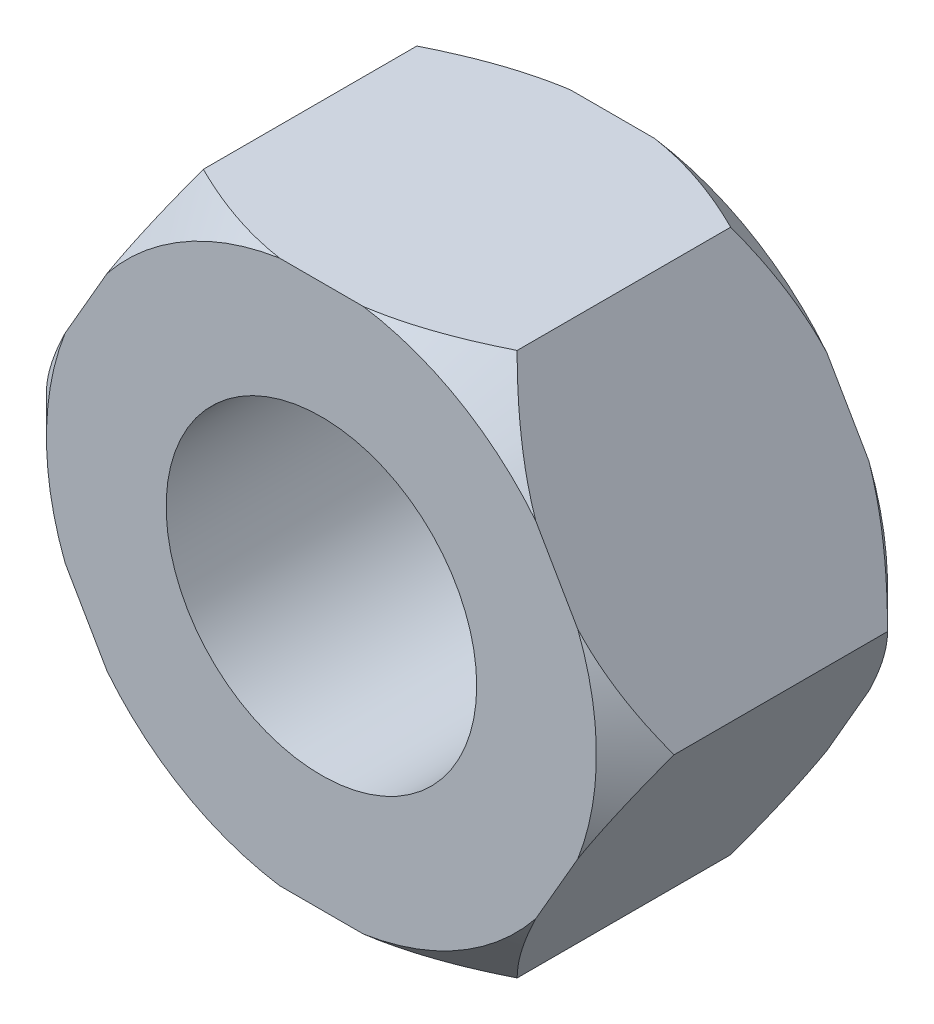
from build123d import *

# Parameters (mm, degrees)
HEX_BODY_15_THICK_DEPTH = 7.5
BORE_PROFILE_16_R       = 8
BORE_16_THRU_DEPTH      = 7.5


with BuildPart() as part:
    # Hex Profile 28 AF → Hex Body 15 Thick (new, symmetric)
    with BuildSketch(Plane.XY):
        Polygon((16.165807537, 0), (8.082903769, 14), (-8.082903769, 14), (-16.165807537, 0), (-8.082903769, -14), (8.082903769, -14), align=None)
    extrude(amount=HEX_BODY_15_THICK_DEPTH, both=True)

    # Bore Profile Ø16 → Bore Ø16 Thru (cut, symmetric)
    with BuildSketch(Plane.XY):
        Circle(BORE_PROFILE_16_R)
    extrude(amount=BORE_16_THRU_DEPTH, both=True, mode=Mode.SUBTRACT)

    # Chamfer Profile 2mm → Double-Sided Chamfer 2mm (revolve, cut)
    with BuildSketch(Plane(origin=(0, 0, 0), x_dir=(1, 0, 0), z_dir=(0, 1, 0))):
        Polygon((16.165807537, 7.5), (16.165807537, 5.5), (14.165807537, 7.5), align=None)
        Polygon((16.165807537, -7.5), (16.165807537, -5.5), (14.165807537, -7.5), align=None)
    revolve(axis=Axis((0, 0, 1000), (0, 0, -1)), mode=Mode.SUBTRACT)


solid = part.part
